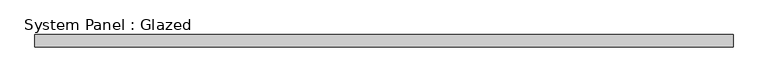
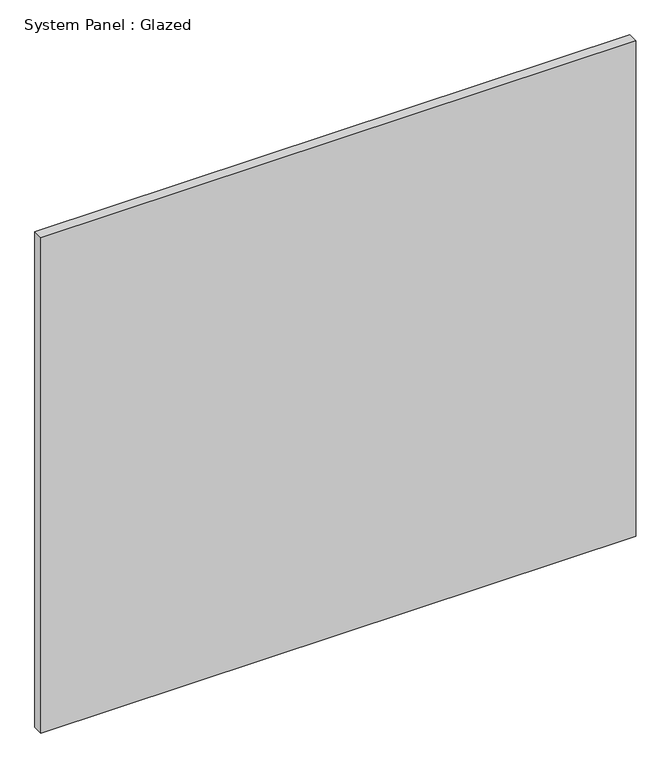
"""IFC4 building model written with IfcOpenShell, lengths in millimetres: plate geometry, System Panel : Glazed."""

from ifc_helpers import new_model, si_unit, origin, origin_with_axes, place, context, project, spatial, polyline, outline, extrude, source, transform, mapped, element, save


def system_panel_glazed_73858ddd(model_context):
    return source(origin(), model_context, "Body", "SweptSolid", [
        extrude(outline(polyline([(727.075, 19.05), (-727.075, 19.05), (-727.075, 44.45), (727.075, 44.45), (727.075, 19.05)])), origin_with_axes(), (0.0, 0.0, 1.0), 1279.4174829),
    ])


if __name__ == "__main__":
    model = new_model("IFC4")
    model_context = context("Model", 3, world=origin())
    ifc_project = project(units=[si_unit("LENGTHUNIT", "METRE", prefix="MILLI")], contexts=[model_context])
    site = spatial("IfcSite", under=ifc_project)
    building = spatial("IfcBuilding", under=site)
    placement = place(None, origin())
    system_panel_glazed_shape = system_panel_glazed_73858ddd(model_context)
    element("IfcPlate", 1, ObjectType="System Panel : Glazed", at=placement, inside=building, context=model_context, shape_type="MappedRepresentation", body=[
        mapped(system_panel_glazed_shape, transform((0.0, 0.0, 0.0), x_axis=(1.0, 0.0, 0.0), y_axis=(0.0, 1.0, 0.0), z_axis=(0.0, 0.0, 1.0))),
    ])
    save(model, "model.ifc")

# Revit data of these elements
# Type "System Panel : Glazed"
#   Construction Type Id = "GSP4R"
#   Analytic Construction = "1/8 in Pilkington single glazing"
#   Visual Light Transmittance = 0.9
#   Solar Heat Gain Coefficient = 0.86
#   Heat Transfer Coefficient (U) = 1.18115 BTU/(h·ft²·°F)
#   Define Thermal Properties by = 1
# Element 1 (IfcPlate, "System Panel : Glazed")
#   Materials on its faces: "Glass"
# Materials
#   "Glass": class "Glass", colour RGB 0 128 192, transparency 0.75, Description = "Soda Lime Glass", Cost = 0
